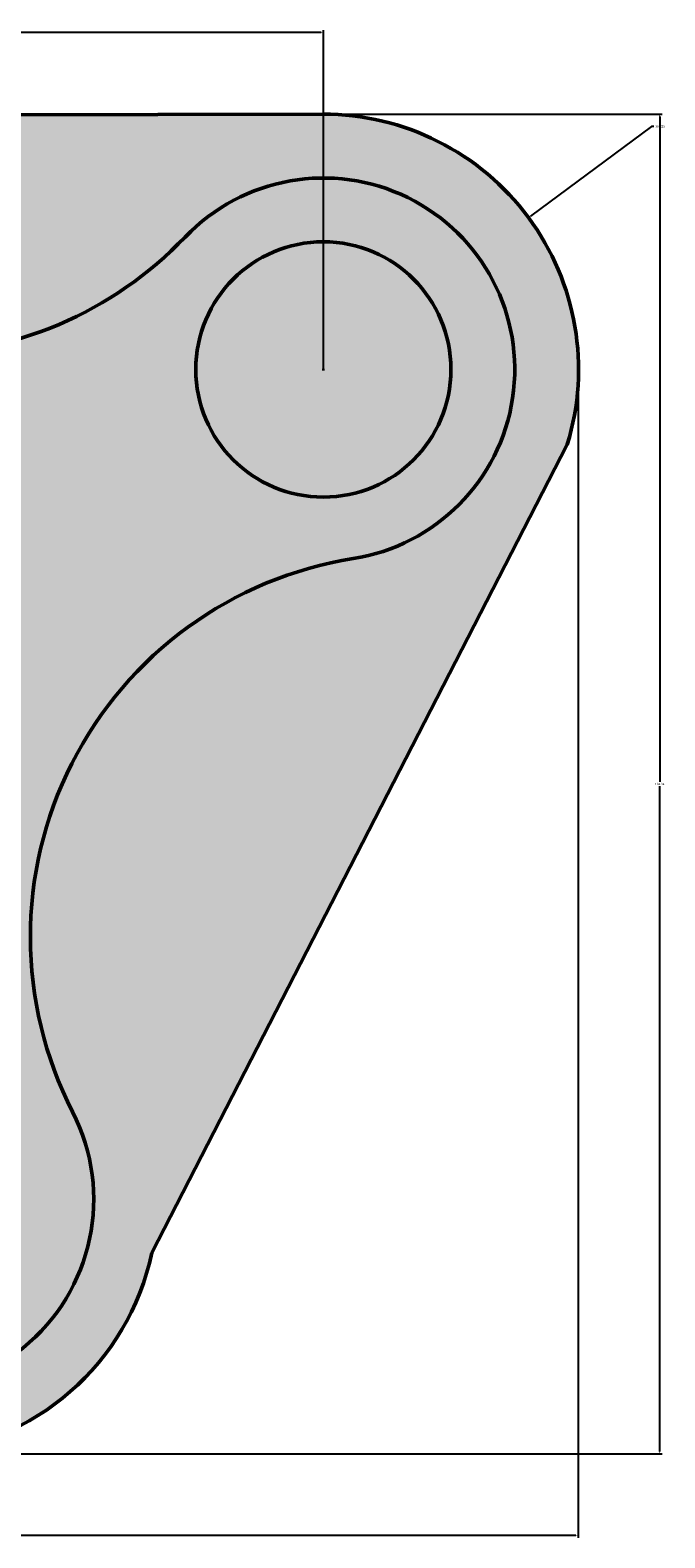
# Model space of a CAD drawing. Units: inches. Extents: x -31 to 87, y -18 to 100.
# Tile 7 of 7: x 37 to 87, y -18 to 100. Entities that reach past the tile are written whole.
import ezdxf

# ---------------------------------------------------------------- set-up
doc = ezdxf.new("R2010")
doc.units = ezdxf.units.IN
doc.header["$MEASUREMENT"] = 0
for name, color, linetype, lineweight in [('M-DIMS', 2, 'Continuous', 18), ('M-HATC', 7, 'Continuous', 18), ('M-OUTL', 4, 'Continuous', 50)]:
    doc.layers.add(name, color=color, linetype=linetype, lineweight=lineweight)
doc.styles.get("Standard").update_dxf_attribs({"font": 'arial.ttf'})
doc.dimstyles.get("Standard").update_dxf_attribs({"dimtxt": 0.18, "dimasz": 0.18, "dimexe": 0.18, "dimexo": 0.0625, "dimgap": 0.09, "dimtad": 0, "dimtih": 1, "dimtoh": 1, "dimdec": 4, "dimzin": 0, "dimdsep": 46, "dimtxsty": 'Standard', "dimcen": 0.09, "dimadec": 0, "dimazin": 0, "dimtfac": 1, "dimtdec": 4, "dimtofl": 0, "dimtmove": 0, "dimatfit": 3, "dimfxl": 1, "dimtolj": 1, "dimtzin": 0, "dimarcsym": 0})

# ---------------------------------------------------------------- blocks, each defined once
blk = doc.blocks.new('*D1')
at = {"layer": 'Defpoints', "color": 0, "transparency": 16777216}
for p in [(-24.62, 75.03), (80.28, 72.24), (80.28, -17.85)]:
    blk.add_point(p, dxfattribs=at)
at = {"layer": 'M-DIMS', "color": 0, "lineweight": -2, "transparency": 16777216}
for p, q in [((-24.62, 74.96), (-24.62, -18.03)), ((80.28, 72.17), (80.28, -18.03)), ((-24.44, -17.85), (27.44, -17.85)), ((80.1, -17.85), (28.21, -17.85))]:
    blk.add_line(p, q, dxfattribs=at)
at = {"layer": 'M-DIMS', "color": 0, "transparency": 16777216}
for points in [[(-24.44, -17.82), (-24.44, -17.88), (-24.62, -17.85)], [(80.1, -17.82), (80.1, -17.88), (80.28, -17.85)]]:
    blk.add_solid(points, dxfattribs=at)
at = {"layer": 'M-DIMS', "color": 0, "transparency": 16777216, "insert": (27.83, -17.85), "char_height": 0.18, "attachment_point": 5}
blk.add_mtext('\\A1;104.9', dxfattribs=at)
blk = doc.blocks.new('*D2')
at = {"layer": 'Defpoints', "color": 0, "transparency": 16777216}
for p in [(60.28, 93.49), (86.68, 93.49), (28.86, -11.45)]:
    blk.add_point(p, dxfattribs=at)
at = {"layer": 'M-DIMS', "color": 0, "lineweight": -2, "transparency": 16777216}
for p, q in [((60.34, 93.49), (86.86, 93.49)), ((86.68, 93.31), (86.68, 41.2)), ((86.68, -11.27), (86.68, 40.84)), ((28.92, -11.45), (86.86, -11.45))]:
    blk.add_line(p, q, dxfattribs=at)
at = {"layer": 'M-DIMS', "color": 0, "transparency": 16777216}
for points in [[(86.65, 93.31), (86.71, 93.31), (86.68, 93.49)], [(86.65, -11.27), (86.71, -11.27), (86.68, -11.45)]]:
    blk.add_solid(points, dxfattribs=at)
at = {"layer": 'M-DIMS', "color": 0, "transparency": 16777216, "insert": (86.68, 41.02), "char_height": 0.18, "attachment_point": 5}
blk.add_mtext('\\A1;104.94', dxfattribs=at)
blk = doc.blocks.new('*D3')
at = {"layer": 'Defpoints', "color": 0, "transparency": 16777216}
for p in [(60.32, 99.89), (-4.68, 73.49), (60.32, 73.49)]:
    blk.add_point(p, dxfattribs=at)
at = {"layer": 'M-DIMS', "color": 0, "lineweight": -2, "transparency": 16777216}
for p, q in [((-4.68, 73.55), (-4.68, 100.07)), ((-4.5, 99.89), (27.6, 99.89)), ((60.14, 99.89), (28.04, 99.89)), ((60.32, 73.55), (60.32, 100.07))]:
    blk.add_line(p, q, dxfattribs=at)
at = {"layer": 'M-DIMS', "color": 0, "transparency": 16777216}
for points in [[(-4.5, 99.92), (-4.5, 99.86), (-4.68, 99.89)], [(60.14, 99.92), (60.14, 99.86), (60.32, 99.89)]]:
    blk.add_solid(points, dxfattribs=at)
at = {"layer": 'M-DIMS', "color": 0, "transparency": 16777216, "insert": (27.82, 99.89), "char_height": 0.18, "attachment_point": 5}
blk.add_mtext('\\A1;65', dxfattribs=at)
blk = doc.blocks.new('*D7')
at = {"layer": 'Defpoints', "color": 0, "transparency": 16777216}
for p in [(76.39, 85.39), (60.32, 73.49)]:
    blk.add_point(p, dxfattribs=at)
at = {"layer": 'M-DIMS', "color": 0, "lineweight": -2, "transparency": 16777216}
for p, q in [((86.04, 92.53), (76.54, 85.5)), ((86.22, 92.53), (86.04, 92.53)), ((60.23, 73.49), (60.41, 73.49)), ((60.32, 73.4), (60.32, 73.58))]:
    blk.add_line(p, q, dxfattribs=at)
at = {"layer": 'M-DIMS', "color": 0, "transparency": 16777216}
blk.add_solid([(76.52, 85.52), (76.56, 85.47), (76.39, 85.39)], dxfattribs=at)
at = {"layer": 'M-DIMS', "color": 0, "transparency": 16777216, "insert": (86.72, 92.53), "char_height": 0.18, "attachment_point": 5}
blk.add_mtext('\\A1;3X R20', dxfattribs=at)

msp = doc.modelspace()

# ---------------------------------------------------------------- hatches: boundary and pattern name
at = {"layer": 'M-HATC'}
h = msp.add_hatch(color=256, dxfattribs=at)
h.set_gradient(color1=(205, 32, 39), color2=(247, 242, 129))
h.paths.add_polyline_path([(-2.425, 93.362, 0.5935038), (-22.614, 64.635), (8.64, 1.342, 0.7463885), (46.874, 4.293), (79.436, 67.614, 0.5051512), (60.278, 93.49)])
h.paths.add_polyline_path([(49.486, 83.865, -1.3922585), (62.663, 58.674, 0.5105468), (40.663, 15.341, -1.6410824), (14.002, 15.393, 0.5052485), (-7.332, 58.726, -1.3771383), (6.152, 83.865, 0.4269308)], flags=16)
h.paths.add_polyline_path([(5.319, 73.49, -1), (-14.681, 73.49, -1)], flags=0)
h.paths.add_polyline_path([(70.319, 73.49, -1), (50.319, 73.49, -1)], flags=0)
h.paths.add_polyline_path([(37.319, 8.49, -1), (17.319, 8.49, -1)], flags=0)
h.paths.add_polyline_path([(6.152, 83.865, 1.3771383), (-7.332, 58.726, -0.5052485), (14.002, 15.393, 1.6410824), (40.663, 15.341, -0.5105468), (62.663, 58.674, 1.3922585), (49.486, 83.865, -0.4269308)], flags=0)
h = msp.add_hatch(color=256, dxfattribs=at)
h.dxf.hatch_style = 1
h.paths.add_polyline_path([(5.319, 73.49, 1), (-14.681, 73.49, 1)])
h.paths.add_polyline_path([(50.319, 73.49, 1), (70.319, 73.49, 1)])
h.paths.add_polyline_path([(37.319, 8.49, 1), (17.319, 8.49, 1)])

# ---------------------------------------------------------------- linework, layer by layer
at = {"layer": 'M-OUTL'}
for p, q in [((-2.425, 93.362), (60.278, 93.49)), ((46.874, 4.293), (79.436, 67.614))]:
    msp.add_line(p, q, dxfattribs=at)
msp.add_circle((60.319, 73.49), 10, dxfattribs=at)
for centre, radius, start, end in [((60.319, 73.49), 20, 342.9139, 90.11661), ((60.319, 73.49), 15, 278.99057, 136.23826), ((27.819, 104.615), 30, 223.76174, 316.23826), ((67.351, 29.043), 30, 98.99057, 207.17632), ((27.319, 8.49), 15, 152.60114, 27.17632), ((27.319, 8.49), 20, 200.93859, 347.88753)]:
    msp.add_arc(centre, radius, start, end, dxfattribs=at)

# ---------------------------------------------------------------- dimensions: what is measured, and where the dimension line sits
at = {"layer": 'M-DIMS'}
for base, p1, p2, override, picture, middle in [((60.319, 99.89), (-4.681, 73.49), (60.319, 73.49), {"dimdec": 0, "dimlfac": 1, "dimrnd": 0, "dimzin": 0, "dimdsep": 46, "dimlunit": 2}, '*D3', (27.819, 99.89)), ((80.28, -17.851), (-24.622, 75.027), (80.28, 72.235), {"dimdec": 1, "dimlfac": 1, "dimrnd": 0, "dimzin": 0, "dimdsep": 46, "dimlunit": 2}, '*D1', (27.829, -17.851))]:
    dim = msp.add_linear_dim(base=base, p1=p1, p2=p2, dimstyle='Standard', override=override, dxfattribs=at)
    dim.commit()
    dim.dimension.update_dxf_attribs({"geometry": picture, "text_midpoint": middle})
dim = msp.add_linear_dim(base=(86.68, 93.49), p1=(28.858, -11.451), p2=(60.278, 93.49), angle=90, dimstyle='Standard', override={"dimdec": 2, "dimlfac": 1, "dimrnd": 0, "dimzin": 0, "dimdsep": 46, "dimlunit": 2}, dxfattribs=at)
dim.commit()
dim.dimension.update_dxf_attribs({"geometry": '*D2', "text_midpoint": (86.68, 41.019)})
dim = msp.add_radius_dim(center=(60.319, 73.49), mpoint=(76.393, 85.391), text='3X <>', dimstyle='Standard', override={"dimdec": 0, "dimlfac": 1, "dimrnd": 0, "dimzin": 0, "dimdsep": 46, "dimlunit": 2}, dxfattribs=at)
dim.commit()
dim.dimension.update_dxf_attribs({"geometry": '*D7', "text_midpoint": (86.715, 92.531), "dimtype": 164})

doc.saveas('drawing.dxf')
